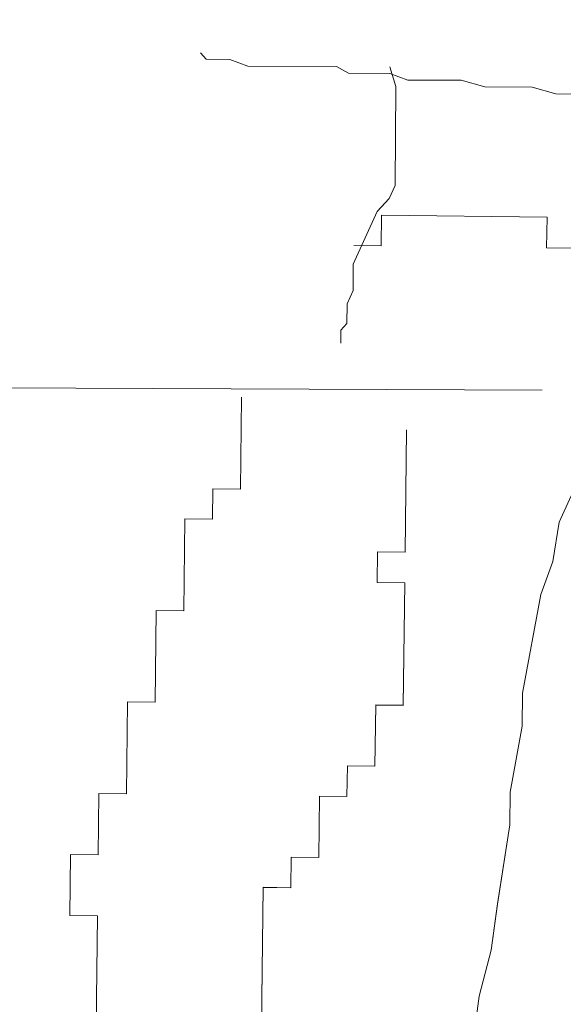
# Model space of a CAD drawing. Units: inches. Extents: x -466983 to 1020, y 324 to 318697.
# Tile 77 of 97: x 650.415 to 652.867, y 944.271 to 948.713. Entities that reach past the tile are written whole.
import ezdxf

# ---------------------------------------------------------------- set-up
doc = ezdxf.new("R2010")
doc.units = ezdxf.units.IN
doc.header["$MEASUREMENT"] = 0
doc.layers.add('A-FLOR-PATT', color=252, linetype='Continuous', lineweight=13)
doc.layers.add('A-FURN', color=8, linetype='Continuous', lineweight=18)

# ---------------------------------------------------------------- blocks, each defined once
blk = doc.blocks.new('L Shaped Sofa')
at = {"ltscale": 2}
for p, q in [((2404.6561, 739.9002), (2404.7023, 743.6789)), ((2402.8786, 740.7957), (2402.9297, 741.175)), ((2406.0202, 740.1355), (2406.0325, 741.1431)), ((2402.7787, 740.4166), (2402.8786, 740.7957)), ((2402.7276, 740.0374), (2402.7787, 740.4166)), ((2406.2471, 740.1327), (2406.0202, 740.1355)), ((2406.2409, 739.6289), (2406.2471, 740.1327)), ((2402.626, 739.3872), (2402.7276, 740.0374)), ((2404.4262, 739.6511), (2404.4293, 739.903)), ((2404.4293, 739.903), (2404.6561, 739.9002)), ((2404.1932, 739.15), (2404.1994, 739.6538)), ((2404.1994, 739.6538), (2404.4262, 739.6511)), ((2406.0079, 739.1279), (2406.0141, 739.6317)), ((2406.0141, 739.6317), (2406.2409, 739.6289)), ((2402.6243, 739.1161), (2402.626, 739.3872)), ((2403.9633, 738.9009), (2403.9664, 739.1528)), ((2403.9664, 739.1528), (2404.1932, 739.15)), ((2405.7718, 738.3749), (2405.7811, 739.1306)), ((2405.7811, 739.1306), (2406.0079, 739.1279)), ((2402.5234, 738.5744), (2402.6243, 739.1161)), ((2403.7303, 738.3998), (2403.7365, 738.9037)), ((2403.7365, 738.9037), (2403.9633, 738.9009)), ((2402.5218, 738.3034), (2402.5234, 738.5744)), ((2403.4912, 737.395), (2403.5035, 738.4026)), ((2403.5035, 738.4026), (2403.7303, 738.3998)), ((2405.5358, 737.6219), (2405.545, 738.3777)), ((2405.545, 738.3777), (2405.7718, 738.3749)), ((2402.3704, 737.4908), (2402.5218, 738.3034)), ((2405.2997, 736.869), (2405.3089, 737.6247)), ((2405.3089, 737.6247), (2405.5358, 737.6219)), ((2402.2712, 737.2202), (2402.3704, 737.4908)), ((2403.718, 737.3922), (2403.4912, 737.395)), ((2403.7149, 737.1403), (2403.718, 737.3922)), ((2402.2204, 736.8951), (2402.2712, 737.2202)), ((2403.4758, 736.1354), (2403.4881, 737.143)), ((2403.4881, 737.143), (2403.7149, 737.1403)), ((2402.1214, 736.6787), (2402.2204, 736.8951)), ((2405.0698, 736.6198), (2405.0729, 736.8717)), ((2405.0729, 736.8717), (2405.2997, 736.869)), ((2404.8337, 735.8669), (2404.843, 736.6226)), ((2404.843, 736.6226), (2405.0698, 736.6198)), ((2402.3601, 735.8101), (2406.8981, 735.7888)), ((2404.0162, 735.3144), (2404.0168, 735.4228)), ((2403.967, 735.2604), (2404.0162, 735.3144)), ((2403.966, 735.0978), (2403.967, 735.2604)), ((2403.9166, 734.9896), (2403.966, 735.0978)), ((2403.9152, 734.7727), (2403.9166, 734.9896)), ((2403.7174, 734.3399), (2403.9152, 734.7727)), ((2402.0963, 734.6406), (2402.3231, 734.6378)), ((2402.3231, 734.6378), (2402.3201, 734.3859)), ((2403.6811, 734.3692), (2403.6842, 734.6212)), ((2403.6842, 734.6212), (2403.911, 734.6184)), ((2402.3201, 734.3859), (2403.6811, 734.3692)), ((2403.6192, 734.2319), (2403.7174, 734.3399)), ((2403.5697, 734.1237), (2403.6192, 734.2319)), ((2403.5647, 733.3105), (2403.5697, 734.1237)), ((2401.7596, 733.3732), (2402.2476, 733.3709)), ((2402.2476, 733.3709), (2402.4424, 733.3157)), ((2402.4424, 733.3157), (2402.8328, 733.3139)), ((2402.8328, 733.3139), (2403.0276, 733.2588)), ((2403.6125, 733.1476), (2403.5647, 733.3105)), ((2403.0276, 733.2588), (2403.4668, 733.2567)), ((2403.4668, 733.2567), (2403.6129, 733.2018)), ((2403.6129, 733.2018), (2403.9544, 733.2002)), ((2403.9544, 733.2002), (2404.0517, 733.1455)), ((2404.0517, 733.1455), (2404.7836, 733.1421)), ((2404.7836, 733.1421), (2404.9297, 733.0872)), ((2404.9297, 733.0872), (2405.1248, 733.0863)), ((2405.1248, 733.0863), (2405.1733, 733.0318))]:
    blk.add_line(p, q, dxfattribs=at)

msp = doc.modelspace()

# ---------------------------------------------------------------- hatches: boundary and pattern name
at = {"layer": 'A-FLOR-PATT', "transparency": 33554572}
h = msp.add_hatch(dxfattribs=at)
h.set_pattern_fill('ANSI37', color=256, scale=30)
h.set_pattern_definition([(45, (-1212.4137, -290.035), (-2.6516504, 2.6516504), []), (135, (-1212.4137, -290.035), (-2.6516504, -2.6516504), [])])
h.paths.add_polyline_path([(901.8057, 1075.9377), (900.6144, 1075.9377), (900.6144, 1065.3856), (899.391, 1065.3856), (898.0911, 1065.3856), (892.8356, 1058.7098, -0.258377), (892.1875, 1058.3509), (879.9848, 1058.3509, -0.20177), (879.4382, 1058.5808), (874.0812, 1065.3856), (872.7813, 1065.3856), (871.5579, 1065.3856), (871.5579, 1075.9377), (813.8057, 1075.9377), (813.8057, 1044.7922), (832.3947, 1044.7922, -0.394795), (848.6602, 1028.5356), (848.6602, 1009.9377), (901.8057, 1009.9377), (901.8057, 1015.9377), (901.3057, 1015.9377), (871.3057, 1015.9377), (871.3057, 1017.2502), (871.3344, 1017.2502, -0.401453), (901.3057, 1045.9377), (901.8057, 1045.9377)])
edge = h.paths.add_edge_path(flags=16)
edge.add_line((847.7731, 1068.9486), (847.7731, 1073.7088))
edge.add_arc((849.2269, 1073.7088), 1.4538, 90, 180, ccw=False)
edge.add_line((849.2269, 1075.1627), (864.4921, 1075.1627))
edge.add_arc((864.4921, 1073.7088), 1.4538, 0, 90, ccw=False)
edge.add_line((865.9459, 1073.7088), (865.9459, 1069.0035))
edge.add_arc((832.6447, 1068.9761), 33.3012, -20.61234, 0.04725, ccw=False)
edge.add_ellipse((856.8595, 1058.48), major_axis=(0, 10.2131), ratio=0.6859192, start_angle=100.00884, end_angle=259.99116, ccw=False)
edge.add_arc((881.0742, 1068.9761), 33.3012, 180.04725, 200.61234, ccw=False)
h.paths.add_polyline_path([(853.1456, 1066.4815), (853.1456, 1066.4534), (853.1463, 1066.4534, 0.433107), (852.9166, 1066.6849), (852.9166, 1066.4534), (853.1456, 1066.4534), (853.1456, 1066.4815), (853.088, 1066.6122, 0.697939), (852.6995, 1066.4534), (852.7003, 1066.4534), (852.7003, 1066.4815), (852.9166, 1067.0012), (852.9166, 1066.6849, -0.396254)], flags=0)
h.paths.add_polyline_path([(861.0187, 1066.4815), (861.0187, 1066.4534), (861.0194, 1066.4534, 0.416404), (860.8024, 1066.6849), (860.8024, 1066.4534), (861.0187, 1066.4534), (861.0187, 1066.4815), (860.9672, 1066.6053, 0.713344), (860.5726, 1066.4534), (860.5734, 1066.4534), (860.5734, 1066.4815), (860.8024, 1067.0012), (860.8024, 1066.6849, -0.379973)], flags=0)
edge = h.paths.add_edge_path(flags=0)
edge.add_spline(control_points=[(861.1298, 1065.7855), (861.4661, 1065.2478), (861.6134, 1065.0161), (861.9833, 1064.3736), (862.1924, 1063.9443), (862.5614, 1063.0391), (862.7212, 1062.5633), (862.9865, 1061.5781), (863.092, 1061.0689), (863.2452, 1060.031), (863.293, 1059.5025), (863.3295, 1058.4409), (863.3181, 1057.9078), (863.2366, 1056.8518), (863.1664, 1056.3289), (862.9695, 1055.308), (862.8427, 1054.8099), (862.5365, 1053.8522), (862.3571, 1053.3927), (861.9514, 1052.5249), (861.7251, 1052.1166), (861.233, 1051.3622), (860.9672, 1051.0162), (860.4048, 1050.3949), (860.1082, 1050.1197), (859.4937, 1049.6461), (859.1758, 1049.4476), (858.5276, 1049.1299), (858.1973, 1049.0107), (857.5315, 1048.8518), (857.1959, 1048.8121), (856.5249, 1048.812), (856.1894, 1048.8515), (855.5236, 1049.0101), (855.1933, 1049.1291), (854.545, 1049.4465), (854.2271, 1049.6449), (853.6124, 1050.1183), (853.3158, 1050.3933), (852.7533, 1051.0143), (852.4874, 1051.3602), (851.9952, 1052.1144), (851.7688, 1052.5225), (851.3629, 1053.3902), (851.1834, 1053.8496), (850.877, 1054.8071), (850.7501, 1055.3051), (850.553, 1056.326), (850.4827, 1056.8488), (850.401, 1057.9048), (850.3895, 1058.4379), (850.4257, 1059.4995), (850.4734, 1060.0281), (850.6265, 1061.066), (850.7318, 1061.5753), (850.9969, 1062.5605), (851.1567, 1063.0365), (851.5254, 1063.9418), (851.7345, 1064.3712), (852.1056, 1065.0164), (852.2544, 1065.2503), (852.6082, 1065.7335)], knot_values=[3.915332, 3.915332, 3.915332, 3.915332, 4.013468, 4.013468, 4.175532, 4.175532, 4.337596, 4.337596, 4.49966, 4.49966, 4.661724, 4.661724, 4.823788, 4.823788, 4.985852, 4.985852, 5.147916, 5.147916, 5.30998, 5.30998, 5.472044, 5.472044, 5.634109, 5.634109, 5.796173, 5.796173, 5.958237, 5.958237, 6.120301, 6.120301, 6.282365, 6.282365, 6.444429, 6.444429, 6.606493, 6.606493, 6.768557, 6.768557, 6.930621, 6.930621, 7.092685, 7.092685, 7.254749, 7.254749, 7.416813, 7.416813, 7.578878, 7.578878, 7.740942, 7.740942, 7.903006, 7.903006, 8.06507, 8.06507, 8.227134, 8.227134, 8.389198, 8.389198, 8.551262, 8.551262, 8.65037, 8.65037, 8.65037, 8.65037], degree=3, periodic=0)
edge.add_line((852.6421, 1065.7855), (861.1298, 1065.7855))
edge = h.paths.add_edge_path(flags=0)
edge.add_ellipse((856.8496, 1057.7432), major_axis=(0, 7.7921), ratio=0.687861, start_angle=0, end_angle=360)
h.paths.add_polyline_path([(848.8634, 1069.3891), (848.8634, 1073.9605, -0.414214), (849.9538, 1075.0508), (863.7652, 1075.0508, -0.414214), (864.8555, 1073.9605), (864.8555, 1069.3891, -0.388936), (864.5237, 1069.027, -0.043561), (849.1953, 1069.027, -0.388936)], flags=0)
h.paths.add_polyline_path([(853.1006, 1068.1122, -1), (852.6775, 1068.1122, -1)], flags=0)
edge = h.paths.add_edge_path(flags=0)
edge.add_ellipse((856.8595, 1057.3378), major_axis=(0, 2.207), ratio=0.657164, start_angle=0, end_angle=360)
h.paths.add_polyline_path([(861.0415, 1068.1122, -1), (860.6184, 1068.1122, -1)], flags=0)
edge = h.paths.add_edge_path()
edge.add_line((573.9537, 1057.3412), (573.9537, 1075.9377))
edge.add_line((573.9537, 1075.9377), (558.7308, 1075.9377))
edge.add_line((558.7308, 1075.9377), (558.7308, 1065.3856))
edge.add_line((558.7308, 1065.3856), (557.5074, 1065.3856))
edge.add_line((557.5074, 1065.3856), (556.2075, 1065.3856))
edge.add_line((556.2075, 1065.3856), (550.952, 1058.7098))
edge.add_arc((550.3039, 1059.1155), 0.7646, 270, 327.9483, ccw=False)
edge.add_line((550.3039, 1058.3509), (538.1012, 1058.3509))
edge.add_arc((538.1012, 1059.1155), 0.7646, 224.3704, 270, ccw=False)
edge.add_line((537.5546, 1058.5808), (532.1976, 1065.3856))
edge.add_line((532.1976, 1065.3856), (530.8977, 1065.3856))
edge.add_line((530.8977, 1065.3856), (529.6743, 1065.3856))
edge.add_line((529.6743, 1065.3856), (529.6743, 1075.9377))
edge.add_line((529.6743, 1075.9377), (520.8057, 1075.9377))
edge.add_line((520.8057, 1075.9377), (520.8057, 1045.9377))
edge.add_line((520.8057, 1045.9377), (521.3057, 1045.9377))
edge.add_arc((521.3057, 1015.9377), 30, 2.50749, 90, ccw=False)
edge.add_line((551.277, 1017.2502), (551.3057, 1017.2502))
edge.add_line((551.3057, 1017.2502), (551.3057, 1015.9377))
edge.add_line((551.3057, 1015.9377), (520.8057, 1015.9377))
edge.add_line((520.8057, 1015.9377), (520.8057, 1009.9377))
edge.add_line((520.8057, 1009.9377), (559.1913, 1010.4022))
edge.add_arc((559.1913, 1011.856), 1.4538, 180, 270, ccw=False)
edge.add_line((557.7375, 1011.856), (557.7375, 1016.5613))
edge.add_arc((591.0386, 1016.5888), 33.3012, 159.38766, 180.04725, ccw=False)
edge.add_ellipse((566.8239, 1027.0848), major_axis=(0, 10.2131), ratio=0.6859192, start_angle=280.00884, end_angle=439.99116, ccw=False)
edge.add_arc((542.6091, 1016.5888), 33.3012, 0.04725, 20.61234, ccw=False)
edge.add_line((575.9103, 1016.6162), (575.9103, 1011.856))
edge.add_arc((574.4565, 1011.856), 1.4538, -90, 0, ccw=False)
edge.add_line((574.4565, 1010.4022), (608.8057, 1009.9377))
edge.add_line((608.8057, 1009.9377), (608.8057, 1041.0857))
edge.add_line((608.8057, 1041.0857), (590.2179, 1041.0857))
edge.add_arc((590.775, 1057.9074), 16.8309, 181.92775, 268.10321, ccw=False)
edge = h.paths.add_edge_path()
edge.add_ellipse((494.2443, 583.6204), major_axis=(0, 10.2131), ratio=0.6859192, start_angle=280.00884, end_angle=439.99116, ccw=False)
edge.add_arc((470.0296, 573.1243), 33.3012, 0.04725, 20.61234, ccw=False)
edge.add_line((503.3307, 573.1518), (503.3307, 568.3916))
edge.add_arc((501.8769, 568.3916), 1.4538, -90, 0, ccw=False)
edge.add_line((501.8769, 566.9377), (539.8057, 566.9377))
edge.add_line((539.8057, 566.9377), (539.8057, 572.9377))
edge.add_line((539.8057, 572.9377), (539.3057, 572.9377))
edge.add_line((539.3057, 572.9377), (509.3057, 572.9377))
edge.add_line((509.3057, 572.9377), (509.3057, 574.2502))
edge.add_line((509.3057, 574.2502), (509.3344, 574.2502))
edge.add_arc((539.3057, 572.9377), 30, 90, 177.49251, ccw=False)
edge.add_line((539.3057, 602.9377), (539.8057, 602.9377))
edge.add_line((539.8057, 602.9377), (539.8057, 626.9377))
edge.add_line((539.8057, 626.9377), (531.7718, 626.9377))
edge.add_line((531.7718, 626.9377), (531.7718, 616.3856))
edge.add_line((531.7718, 616.3856), (530.5484, 616.3856))
edge.add_line((530.5484, 616.3856), (529.2485, 616.3856))
edge.add_line((529.2485, 616.3856), (523.7105, 609.3509))
edge.add_line((523.7105, 609.3509), (510.7766, 609.3509))
edge.add_line((510.7766, 609.3509), (505.2386, 616.3856))
edge.add_line((505.2386, 616.3856), (503.9387, 616.3856))
edge.add_line((503.9387, 616.3856), (502.7153, 616.3856))
edge.add_line((502.7153, 616.3856), (502.7153, 626.9377))
edge.add_line((502.7153, 626.9377), (481.6983, 626.9377))
edge.add_line((481.6983, 626.9377), (481.6983, 610.995))
edge.add_arc((467.2703, 611.4728), 14.4359, 271.92775, 358.10321, ccw=False)
edge.add_line((467.7559, 597.0451), (451.8057, 597.0451))
edge.add_line((451.8057, 597.0451), (451.8057, 584.4035))
edge.add_line((451.8057, 584.4035), (451.8057, 566.9377))
edge.add_line((451.8057, 566.9377), (486.6117, 566.9377))
edge.add_arc((486.6117, 568.3916), 1.4538, 180, 270, ccw=False)
edge.add_line((485.1579, 568.3916), (485.1579, 573.0969))
edge.add_arc((518.4591, 573.1243), 33.3012, 159.38766, 180.04725, ccw=False)
h.paths.add_polyline_path([(836.2609, 1020.7328), (879.8898, 1020.7328), (879.8898, 1039.3902), (836.2609, 1039.3902)], flags=25)
h.paths.add_polyline_path([(549.9851, 1036.7492), (593.614, 1036.7492), (593.614, 1055.4065), (549.9851, 1055.4065)], flags=24)
h.paths.add_polyline_path([(475.123, 595.5959), (518.752, 595.5959), (518.752, 614.2532), (475.123, 614.2532)], flags=24)
h = msp.add_hatch(dxfattribs=at)
h.set_pattern_fill('ANSI37', color=256, scale=20)
h.set_pattern_definition([(45, (-1212.4137, -290.035), (-1.767767, 1.767767), []), (135, (-1212.4137, -290.035), (-1.767767, -1.767767), [])])
h.paths.add_polyline_path([(809.8057, 870.9377), (809.8057, 888.1519), (806.9985, 888.1519), (802.6624, 888.1519), (789.3832, 888.1519), (786.2846, 888.1519, -0.414214), (785.4991, 888.9374), (785.4991, 900.1959), (785.4991, 908.4696, -0.414214), (786.8082, 909.7787, -0.414214), (785.4991, 911.0878), (785.4991, 929.1015, -0.414214), (786.8082, 930.4106, -0.414214), (785.4991, 931.7197), (785.4991, 931.9039, -0.414214), (784.19, 930.5948), (766.7223, 930.5948, -0.412359), (765.4132, 931.8956, -0.413741), (764.1145, 930.5782), (744.5781, 930.422, -0.416556), (743.7864, 931.2075), (743.7864, 933.5153), (742.2154, 933.5153), (742.2154, 952.024, -0.001344), (743.7864, 952.1998), (743.7864, 953.9377), (678.5915, 953.9377), (678.5915, 951.1305), (678.5915, 946.7945), (678.5915, 933.5153), (678.5915, 930.4166, -0.414214), (677.806, 929.6312), (666.5475, 929.6312), (658.2738, 929.6312, -0.414214), (656.9647, 930.9403, -0.414214), (655.6556, 929.6312), (637.6419, 929.6312, -0.414214), (636.3328, 930.9403, -0.414214), (635.0237, 929.6312), (634.8395, 929.6312, -0.414214), (636.1486, 928.322), (636.1486, 910.8544, -0.412359), (634.8478, 909.5452, -0.413741), (636.1653, 908.2466), (636.3214, 888.7102, -0.416556), (635.5359, 887.9184), (633.2281, 887.9184), (633.2281, 886.3475), (614.7194, 886.3475, -0.001344), (614.5436, 887.9184), (612.8057, 887.9184), (612.8057, 834.9377), (612.8057, 752.9377), (612.8057, 748.9377), (612.8057, 697.9377), (654.8057, 697.9377), (654.8057, 701.9377), (715.8057, 701.9377), (715.8057, 737.4353), (774.2918, 737.4353), (774.2918, 795.9377), (809.8057, 795.9377)])
h.paths.add_polyline_path([(679.2761, 849.5757, 0.102523), (682.1475, 849.2608, -0.080461), (694.5428, 849.7725, -0.283899), (694.4822, 849.0082, 0.136605), (694.4068, 848.8103, -0.030441), (694.5428, 846.8929), (694.5428, 842.6198), (694.5428, 838.3466, -0.028219), (694.4246, 836.5684), (694.425, 836.5684, 0.196187), (694.4456, 836.2708, -0.302897), (694.5428, 835.467, -0.080461), (682.1475, 835.9787, 0.102523), (679.2761, 835.6638, -0.58611), (678.6457, 836.0169), (678.6457, 849.2227, -0.58611)], flags=16)
h.paths.add_polyline_path([(679.5173, 848.6515, 0.699597), (679.476, 848.6342, 1.20716), (679.1935, 848.7422, 0.010621)], flags=0)
h.paths.add_polyline_path([(679.4923, 836.5608, -0.013798), (679.9178, 836.6594, -0.071703), (682.8533, 837.1434, -0.165743), (682.1665, 839.1006), (682.1665, 842.6094), (682.1665, 846.0603, -0.240616), (683.4733, 848.6767, -0.068263), (693.9295, 849.0082), (693.7875, 848.7083), (693.7875, 849.0228, 0.067332), (683.4733, 848.6767, 0.240616), (682.1665, 846.0603), (682.1665, 842.6094), (682.1665, 839.1006, 0.23459), (683.461, 836.5513, 0.068093), (693.7875, 836.1955), (693.7875, 836.5104), (693.9296, 836.2102, -0.077215), (682.2421, 836.7815, 0.086627), (679.5283, 836.5701, -0.628402), (679.5029, 836.5735), (679.5029, 836.6071, 0.910458)], flags=0)
h.paths.add_polyline_path([(679.476, 848.6364), (679.2069, 848.647), (679.2069, 836.5718, 0.913566), (679.3645, 836.5861), (679.476, 836.5824)], flags=0)
h.paths.add_polyline_path([(679.2761, 829.8604, 0.102523), (682.1475, 829.5455, -0.080461), (694.5428, 830.0572, -0.283899), (694.4822, 829.2929, 0.136605), (694.4068, 829.095, -0.030441), (694.5428, 827.1776), (694.5428, 822.9045), (694.5428, 818.6314, -0.028219), (694.4246, 816.8531), (694.425, 816.8532, 0.196187), (694.4456, 816.5555, -0.302897), (694.5428, 815.7517, -0.080461), (682.1475, 816.2635, 0.102523), (679.2761, 815.9485, -0.58611), (678.6457, 816.3016), (678.6457, 829.5074, -0.58611)], flags=16)
h.paths.add_polyline_path([(679.5173, 828.9362, 0.699597), (679.476, 828.9189, 1.20716), (679.1935, 829.0269, 0.010621)], flags=0)
h.paths.add_polyline_path([(679.4923, 816.8456, -0.013798), (679.9178, 816.9441, -0.071703), (682.8533, 817.4281, -0.165743), (682.1665, 819.3853), (682.1665, 822.8941), (682.1665, 826.345, -0.240616), (683.4733, 828.9614, -0.068263), (693.9295, 829.2929), (693.7875, 828.9931), (693.7875, 829.3076, 0.067332), (683.4733, 828.9614, 0.240616), (682.1665, 826.345), (682.1665, 822.8941), (682.1665, 819.3853, 0.23459), (683.461, 816.836, 0.068093), (693.7875, 816.4802), (693.7875, 816.7952), (693.9296, 816.4949, -0.077215), (682.2421, 817.0662, 0.086627), (679.5283, 816.8549, -0.628402), (679.5029, 816.8582), (679.5029, 816.8918, 0.910458)], flags=0)
h.paths.add_polyline_path([(679.476, 828.9211), (679.2069, 828.9317), (679.2069, 816.8565, 0.913566), (679.3645, 816.8708), (679.476, 816.8671)], flags=0)
h.paths.add_polyline_path([(679.2761, 810.1451, 0.102523), (682.1475, 809.8302, -0.080461), (694.5428, 810.342, -0.3023), (694.4466, 809.5394, 0.10023), (694.4058, 809.3878, -0.03057), (694.5428, 807.4623), (694.5428, 803.1892), (694.5428, 798.9161, -0.03057), (694.4058, 796.9906, 0.10023), (694.4466, 796.839, -0.3023), (694.5428, 796.0365, -0.080461), (682.1475, 796.5482, 0.102523), (679.2761, 796.2333, -0.58611), (678.6457, 796.5863), (678.6457, 809.7921, -0.58611)], flags=16)
h.paths.add_polyline_path([(679.5173, 809.2417, 0.699597), (679.476, 809.2244, 1.20716), (679.1935, 809.3324, 0.010621)], flags=0)
h.paths.add_polyline_path([(679.4923, 797.151, -0.013798), (679.9178, 797.2496, -0.071703), (682.8533, 797.7336, -0.165743), (682.1665, 799.6908), (682.1665, 803.1996), (682.1665, 806.6505, -0.239349), (683.461, 809.2577, -0.072465), (694.4468, 809.5405, 0.197932), (694.425, 809.2405), (693.7875, 809.2985), (693.7875, 809.6135, 0.068093), (683.461, 809.2577, 0.239349), (682.1665, 806.6505), (682.1665, 803.1996), (682.1665, 799.6908, 0.235854), (683.4733, 797.1323, 0.067332), (693.7875, 796.7861), (693.7875, 797.1006), (694.425, 797.1586, 0.197932), (694.4468, 796.8586, -0.080419), (682.1557, 797.3795, 0.083867), (679.5283, 797.1603, -0.628402), (679.5029, 797.1637), (679.5029, 797.1973, 0.910458)], flags=0)
h.paths.add_polyline_path([(679.2069, 809.2372), (679.2069, 797.162, 0.913566), (679.3645, 797.1763), (679.476, 797.1726), (679.476, 809.2266)], flags=0)
h.paths.add_polyline_path([(695.3643, 853.2989), (728.2231, 853.2989), (728.2231, 771.1519), (695.3643, 771.1519)], flags=16)
h.paths.add_polyline_path([(696.0215, 852.6417), (727.5659, 852.6417), (727.5659, 771.809), (696.0215, 771.809)], flags=0)
h.paths.add_polyline_path([(679.2761, 788.7869, 0.102523), (682.1475, 788.472, -0.080461), (694.5428, 788.9837, -0.3023), (694.4466, 788.1812, 0.10023), (694.4058, 788.0296, -0.03057), (694.5428, 786.1041), (694.5428, 781.831), (694.5428, 777.5578, -0.03057), (694.4058, 775.6323, 0.10023), (694.4466, 775.4808, -0.3023), (694.5428, 774.6782, -0.080461), (682.1475, 775.19, 0.102523), (679.2761, 774.875, -0.58611), (678.6457, 775.2281), (678.6457, 788.4339, -0.58611)], flags=16)
h.paths.add_polyline_path([(679.5173, 787.8834, 0.699597), (679.476, 787.8662, 1.20716), (679.1935, 787.9742, 0.010621)], flags=0)
h.paths.add_polyline_path([(679.4923, 775.7928, -0.013798), (679.9178, 775.8914, -0.071703), (682.8533, 776.3753, -0.165743), (682.1665, 778.3325), (682.1665, 781.8414), (682.1665, 785.2922, -0.239349), (683.461, 787.8995, -0.072465), (694.4468, 788.1823, 0.197932), (694.425, 787.8823), (693.7875, 787.9403), (693.7875, 788.2553, 0.068093), (683.461, 787.8995, 0.239349), (682.1665, 785.2922), (682.1665, 781.8414), (682.1665, 778.3325, 0.235854), (683.4733, 775.7741, 0.067332), (693.7875, 775.4279), (693.7875, 775.7424), (694.425, 775.8004, 0.197932), (694.4468, 775.5004, -0.080419), (682.1557, 776.0212, 0.083867), (679.5283, 775.8021, -0.628402), (679.5029, 775.8054), (679.5029, 775.8391, 0.910458)], flags=0)
h.paths.add_polyline_path([(679.2069, 787.8789), (679.2069, 775.8038, 0.913566), (679.3645, 775.818), (679.476, 775.8144), (679.476, 787.8684)], flags=0)
h.paths.add_polyline_path([(704.641, 854.1204, -0.080461), (705.1527, 866.5157, 0.102523), (704.8378, 869.3871, -0.58611), (705.1908, 870.0174), (718.3966, 870.0174, -0.58611), (718.7496, 869.3871, 0.102523), (718.4347, 866.5157, -0.080461), (718.9465, 854.1204, -0.3023), (718.1439, 854.2166, 0.10023), (717.9924, 854.2574, -0.03057), (716.0668, 854.1204), (711.7937, 854.1204), (707.5206, 854.1204, -0.03057), (705.5951, 854.2574, 0.10023), (705.4435, 854.2166, -0.3023)], flags=16)
h.paths.add_polyline_path([(717.8462, 869.1459, 0.699597), (717.8289, 869.1872, 1.20716), (717.9369, 869.4697, 0.010621)], flags=0)
h.paths.add_polyline_path([(705.4631, 854.2164, -0.080419), (705.984, 866.5074, 0.083867), (705.7648, 869.1349, -0.628402), (705.7682, 869.1603), (705.8018, 869.1603, 0.910458), (705.7555, 869.1709, -0.013798), (705.8541, 868.7454, -0.071703), (706.3381, 865.8099, -0.165743), (708.2953, 866.4967), (711.8041, 866.4967), (715.255, 866.4967, -0.239349), (717.8622, 865.2022, -0.072465), (718.145, 854.2164, 0.197932), (717.845, 854.2382), (717.903, 854.8757), (718.218, 854.8757, 0.068093), (717.8622, 865.2022, 0.239349), (715.255, 866.4967), (711.8041, 866.4967), (708.2953, 866.4967, 0.235854), (705.7368, 865.1898, 0.067332), (705.3906, 854.8757), (705.7051, 854.8757), (705.7631, 854.2382, 0.197932)], flags=16)
h.paths.add_polyline_path([(705.7665, 869.4563, 0.913566), (705.7808, 869.2987), (705.7771, 869.1872), (717.8311, 869.1872), (717.8417, 869.4563)], flags=0)
h.paths.add_polyline_path([(729.0446, 842.6198), (729.0446, 846.8929, -0.03057), (729.1817, 848.8184, 0.10023), (729.1408, 848.9699, -0.3023), (729.0446, 849.7725, -0.080461), (741.4399, 849.2608, 0.102523), (744.3113, 849.5757, -0.58611), (744.9417, 849.2227), (744.9417, 836.0169, -0.58611), (744.3113, 835.6638, 0.102523), (741.4399, 835.9787, -0.080461), (729.0446, 835.467, -0.3023), (729.1408, 836.2696, 0.10023), (729.1817, 836.4211, -0.03057), (729.0446, 838.3466)], flags=16)
h.paths.add_polyline_path([(744.1115, 836.5846, 1.20716), (744.3939, 836.4766, 0.010621), (744.0701, 836.5673, 0.699597)], flags=0)
h.paths.add_polyline_path([(729.1407, 836.2684, 0.197932), (729.1624, 836.5684), (729.7999, 836.5104), (729.7999, 836.1955, 0.068093), (740.1264, 836.5513, 0.239349), (741.4209, 839.1585), (741.4209, 842.6094), (741.4209, 846.1182, 0.235854), (740.1141, 848.6767, 0.067332), (729.7999, 849.0228), (729.7999, 848.7083), (729.1624, 848.6503, 0.197932), (729.1407, 848.9504, -0.080419), (741.4317, 848.4295, 0.083867), (744.0591, 848.6486, -0.628402), (744.0845, 848.6453), (744.0845, 848.6117, 0.910458), (744.0951, 848.6579, -0.013798), (743.6696, 848.5594, -0.071703), (740.7341, 848.0754, -0.165743), (741.4209, 846.1182), (741.4209, 842.6094), (741.4209, 839.1585, -0.239349), (740.1264, 836.5513, -0.072465)], flags=0)
h.paths.add_polyline_path([(729.0446, 830.0572, -0.080461), (741.4399, 829.5455, 0.102523), (744.3113, 829.8604, -0.58611), (744.9417, 829.5074), (744.9417, 816.3016, -0.58611), (744.3113, 815.9485, 0.102523), (741.4399, 816.2635, -0.080461), (729.0446, 815.7517, -0.3023), (729.1408, 816.5543, 0.10023), (729.1817, 816.7058, -0.03057), (729.0446, 818.6314), (729.0446, 822.9045), (729.0446, 827.1776, -0.03057), (729.1817, 829.1031, 0.10023), (729.1408, 829.2547, -0.3023)], flags=16)
h.paths.add_polyline_path([(744.1115, 816.8693, 1.20716), (744.3939, 816.7613, 0.010621), (744.0701, 816.852, 0.699597)], flags=0)
h.paths.add_polyline_path([(729.1407, 829.2351, -0.080419), (741.4317, 828.7142, 0.083867), (744.0591, 828.9334, -0.628402), (744.0845, 828.93), (744.0845, 828.8964, 0.910458), (744.0951, 828.9427, -0.013798), (743.6696, 828.8441, -0.071703), (740.7341, 828.3601, -0.165743), (741.4209, 826.4029), (741.4209, 822.8941), (741.4209, 819.4432, -0.239349), (740.1264, 816.836, -0.072465), (729.1407, 816.5531, 0.197932), (729.1624, 816.8532), (729.7999, 816.7952), (729.7999, 816.4802, 0.068093), (740.1264, 816.836, 0.239349), (741.4209, 819.4432), (741.4209, 822.8941), (741.4209, 826.4029, 0.235854), (740.1141, 828.9614, 0.067332), (729.7999, 829.3076), (729.7999, 828.9931), (729.1624, 828.9351, 0.197932)], flags=16)
h.paths.add_polyline_path([(729.0446, 810.342, -0.080461), (741.4399, 809.8302, 0.102523), (744.3113, 810.1451, -0.58611), (744.9417, 809.7921), (744.9417, 796.5863, -0.58611), (744.3113, 796.2333, 0.102523), (741.4399, 796.5482, -0.080461), (729.0446, 796.0365, -0.283899), (729.1052, 796.8007, 0.136605), (729.1806, 796.9987, -0.030441), (729.0446, 798.9161), (729.0446, 803.1892), (729.0446, 807.4623, -0.028219), (729.1628, 809.2406), (729.1624, 809.2405, 0.196187), (729.1418, 809.5382, -0.302897)], flags=16)
h.paths.add_polyline_path([(744.1115, 797.1748, 1.20716), (744.3939, 797.0668, 0.010621), (744.0701, 797.1575, 0.699597)], flags=0)
h.paths.add_polyline_path([(741.3453, 809.0275, 0.086627), (744.0591, 809.2388, -0.628402), (744.0845, 809.2355), (744.0845, 809.2019, 0.910458), (744.0951, 809.2481, -0.013798), (743.6696, 809.1496, -0.071703), (740.7341, 808.6656, -0.165743), (741.4209, 806.7084), (741.4209, 803.1996), (741.4209, 799.7487, -0.240616), (740.1141, 797.1323, -0.068263), (729.658, 796.8008), (729.7999, 797.1006), (729.7999, 796.7861, 0.067332), (740.1141, 797.1323, 0.240616), (741.4209, 799.7487), (741.4209, 803.1996), (741.4209, 806.7084, 0.23459), (740.1264, 809.2577, 0.068093), (729.7999, 809.6135), (729.7999, 809.2985), (729.6578, 809.5988, -0.077215)], flags=0)
h.paths.add_polyline_path([(704.641, 770.3304, -0.283899), (705.4053, 770.2697, 0.136605), (705.6032, 770.1944, -0.030441), (707.5206, 770.3304), (711.7937, 770.3304), (716.0668, 770.3304, -0.028219), (717.8451, 770.2122), (717.845, 770.2126, 0.196187), (718.1427, 770.2331, -0.302897), (718.9465, 770.3304, -0.080461), (718.4347, 757.9351, 0.102523), (718.7496, 755.0637, -0.58611), (718.3966, 754.4333), (705.1908, 754.4333, -0.58611), (704.8378, 755.0637, 0.102523), (705.1527, 757.9351, -0.080461)], flags=16)
h.paths.add_polyline_path([(705.762, 755.3048, 0.699597), (705.7793, 755.2635, 1.20716), (705.6713, 754.9811, 0.010621)], flags=0)
h.paths.add_polyline_path([(705.4053, 769.717), (705.7051, 769.5751), (705.3906, 769.5751, 0.067332), (705.7368, 759.2609, 0.240616), (708.3532, 757.954), (711.8041, 757.954), (715.3129, 757.954, 0.23459), (717.8622, 759.2485, 0.068093), (718.218, 769.5751), (717.903, 769.5751), (718.2033, 769.7172, -0.077215), (717.632, 758.0297, 0.086627), (717.8433, 755.3159, -0.628402), (717.84, 755.2904), (717.8064, 755.2904, 0.910458), (717.8526, 755.2799, -0.013798), (717.7541, 755.7053, -0.071703), (717.2701, 758.6409, -0.165743), (715.3129, 757.954), (711.8041, 757.954), (708.3532, 757.954, -0.240616), (705.7368, 759.2609, -0.068263)], flags=0)
h.paths.add_polyline_path([(729.0446, 788.9837, -0.080461), (741.4399, 788.472, 0.102523), (744.3113, 788.7869, -0.58611), (744.9417, 788.4339), (744.9417, 775.2281, -0.58611), (744.3113, 774.875, 0.102523), (741.4399, 775.19, -0.080461), (729.0446, 774.6782, -0.283899), (729.1052, 775.4425, 0.136605), (729.1806, 775.6405, -0.030441), (729.0446, 777.5578), (729.0446, 781.831), (729.0446, 786.1041, -0.028219), (729.1628, 787.8823), (729.1624, 787.8823, 0.196187), (729.1418, 788.1799, -0.302897)], flags=16)
h.paths.add_polyline_path([(744.1115, 775.8165, 1.20716), (744.3939, 775.7086, 0.010621), (744.0701, 775.7993, 0.699597)], flags=0)
h.paths.add_polyline_path([(741.3453, 787.6692, 0.086627), (744.0591, 787.8806, -0.628402), (744.0845, 787.8773), (744.0845, 787.8437, 0.910458), (744.0951, 787.8899, -0.013798), (743.6696, 787.7913, -0.071703), (740.7341, 787.3074, -0.165743), (741.4209, 785.3502), (741.4209, 781.8414), (741.4209, 778.3905, -0.240616), (740.1141, 775.7741, -0.068263), (729.658, 775.4425), (729.7999, 775.7424), (729.7999, 775.4279, 0.067332), (740.1141, 775.7741, 0.240616), (741.4209, 778.3905), (741.4209, 781.8414), (741.4209, 785.3502, 0.23459), (740.1264, 787.8995, 0.068093), (729.7999, 788.2553), (729.7999, 787.9403), (729.6578, 788.2405, -0.077215)], flags=0)
h.paths.add_polyline_path([(744.1115, 848.6364), (744.1115, 836.5824), (744.3805, 836.5718), (744.3805, 848.647, 0.913566), (744.2229, 848.6327)], flags=0)
h.paths.add_polyline_path([(744.2229, 828.9174), (744.1115, 828.9211), (744.1115, 816.8671), (744.3805, 816.8565), (744.3805, 828.9317, 0.913566)], flags=0)
h.paths.add_polyline_path([(717.8311, 755.2635), (705.7771, 755.2635), (705.7665, 754.9945), (717.8417, 754.9945, 0.913566), (717.8274, 755.1521)], flags=0)
h.paths.add_polyline_path([(744.2229, 809.2229), (744.1115, 809.2266), (744.1115, 797.1726), (744.3805, 797.162), (744.3805, 809.2372, 0.913566)], flags=0)
h.paths.add_polyline_path([(744.1115, 787.8684), (744.1115, 775.8144), (744.3805, 775.8038), (744.3805, 787.8789, 0.913566), (744.2229, 787.8647)], flags=0)
h.paths.add_polyline_path([(678.8774, 877.1228), (737.6127, 877.1228), (737.6127, 899.5116), (678.8774, 899.5116)], flags=24)

# ---------------------------------------------------------------- linework, layer by layer
at = {"layer": 'A-FURN', "ltscale": 2}
for p, q in [((651.2564, 948.534), (651.2298, 948.5639)), ((651.2564, 948.534), (651.2298, 948.5639)), ((651.2564, 948.534), (651.2298, 948.5639)), ((651.2564, 948.534), (651.2298, 948.5639)), ((651.2564, 948.534), (651.2298, 948.5639)), ((651.2564, 948.534), (651.2298, 948.5639)), ((651.3634, 948.5335), (651.2564, 948.534)), ((651.3634, 948.5335), (651.2564, 948.534)), ((651.3634, 948.5335), (651.2564, 948.534)), ((651.3634, 948.5335), (651.2564, 948.534)), ((651.3634, 948.5335), (651.2564, 948.534)), ((651.3634, 948.5335), (651.2564, 948.534)), ((651.4435, 948.5034), (651.3634, 948.5335)), ((651.4435, 948.5034), (651.3634, 948.5335)), ((651.4435, 948.5034), (651.3634, 948.5335)), ((651.4435, 948.5034), (651.3634, 948.5335)), ((651.4435, 948.5034), (651.3634, 948.5335)), ((651.4435, 948.5034), (651.3634, 948.5335)), ((651.8447, 948.5016), (651.4435, 948.5034)), ((651.8447, 948.5016), (651.4435, 948.5034)), ((651.8447, 948.5016), (651.4435, 948.5034)), ((651.8447, 948.5016), (651.4435, 948.5034)), ((651.8447, 948.5016), (651.4435, 948.5034)), ((651.8447, 948.5016), (651.4435, 948.5034)), ((651.898, 948.4716), (651.8447, 948.5016)), ((651.898, 948.4716), (651.8447, 948.5016)), ((651.898, 948.4716), (651.8447, 948.5016)), ((651.898, 948.4716), (651.8447, 948.5016)), ((651.898, 948.4716), (651.8447, 948.5016)), ((651.898, 948.4716), (651.8447, 948.5016)), ((652.0855, 948.5004), (652.1117, 948.4111)), ((652.0855, 948.5004), (652.1117, 948.4111)), ((652.0855, 948.5004), (652.1117, 948.4111)), ((652.0855, 948.5004), (652.1117, 948.4111)), ((652.0855, 948.5004), (652.1117, 948.4111)), ((652.0855, 948.5004), (652.1117, 948.4111)), ((652.0853, 948.4707), (651.898, 948.4716)), ((652.0853, 948.4707), (651.898, 948.4716)), ((652.0853, 948.4707), (651.898, 948.4716)), ((652.0853, 948.4707), (651.898, 948.4716)), ((652.0853, 948.4707), (651.898, 948.4716)), ((652.0853, 948.4707), (651.898, 948.4716)), ((652.1654, 948.4406), (652.0853, 948.4707)), ((652.1654, 948.4406), (652.0853, 948.4707)), ((652.1654, 948.4406), (652.0853, 948.4707)), ((652.1654, 948.4406), (652.0853, 948.4707)), ((652.1654, 948.4406), (652.0853, 948.4707)), ((652.1654, 948.4406), (652.0853, 948.4707)), ((652.1117, 948.4111), (652.1089, 947.9653)), ((652.1117, 948.4111), (652.1089, 947.9653)), ((652.1117, 948.4111), (652.1089, 947.9653)), ((652.1117, 948.4111), (652.1089, 947.9653)), ((652.1117, 948.4111), (652.1089, 947.9653)), ((652.1117, 948.4111), (652.1089, 947.9653)), ((652.4061, 948.4395), (652.1654, 948.4406)), ((652.4061, 948.4395), (652.1654, 948.4406)), ((652.4061, 948.4395), (652.1654, 948.4406)), ((652.4061, 948.4395), (652.1654, 948.4406)), ((652.4061, 948.4395), (652.1654, 948.4406)), ((652.4061, 948.4395), (652.1654, 948.4406)), ((652.5129, 948.4093), (652.4061, 948.4395)), ((652.5129, 948.4093), (652.4061, 948.4395)), ((652.5129, 948.4093), (652.4061, 948.4395)), ((652.5129, 948.4093), (652.4061, 948.4395)), ((652.5129, 948.4093), (652.4061, 948.4395)), ((652.5129, 948.4093), (652.4061, 948.4395)), ((652.7269, 948.4083), (652.5129, 948.4093)), ((652.7269, 948.4083), (652.5129, 948.4093)), ((652.7269, 948.4083), (652.5129, 948.4093)), ((652.7269, 948.4083), (652.5129, 948.4093)), ((652.7269, 948.4083), (652.5129, 948.4093)), ((652.7269, 948.4083), (652.5129, 948.4093)), ((652.8337, 948.378), (652.7269, 948.4083)), ((652.8337, 948.378), (652.7269, 948.4083)), ((652.8337, 948.378), (652.7269, 948.4083)), ((652.8337, 948.378), (652.7269, 948.4083)), ((652.8337, 948.378), (652.7269, 948.4083)), ((652.8337, 948.378), (652.7269, 948.4083)), ((653.1012, 948.3768), (652.8337, 948.378)), ((653.1012, 948.3768), (652.8337, 948.378)), ((653.1012, 948.3768), (652.8337, 948.378)), ((653.1012, 948.3768), (652.8337, 948.378)), ((653.1012, 948.3768), (652.8337, 948.378)), ((653.1012, 948.3768), (652.8337, 948.378)), ((652.1089, 947.9653), (652.0818, 947.906)), ((652.1089, 947.9653), (652.0818, 947.906)), ((652.1089, 947.9653), (652.0818, 947.906)), ((652.1089, 947.9653), (652.0818, 947.906)), ((652.1089, 947.9653), (652.0818, 947.906)), ((652.1089, 947.9653), (652.0818, 947.906)), ((652.0818, 947.906), (652.028, 947.8468)), ((652.0818, 947.906), (652.028, 947.8468)), ((652.0818, 947.906), (652.028, 947.8468)), ((652.0818, 947.906), (652.028, 947.8468)), ((652.0818, 947.906), (652.028, 947.8468)), ((652.0818, 947.906), (652.028, 947.8468)), ((652.028, 947.8468), (651.9195, 947.6095)), ((652.028, 947.8468), (651.9195, 947.6095)), ((652.028, 947.8468), (651.9195, 947.6095)), ((652.028, 947.8468), (651.9195, 947.6095)), ((652.028, 947.8468), (651.9195, 947.6095)), ((652.028, 947.8468), (651.9195, 947.6095)), ((652.0479, 947.8307), (652.0462, 947.6926)), ((652.0479, 947.8307), (652.0462, 947.6926)), ((652.0479, 947.8307), (652.0462, 947.6926)), ((652.0479, 947.8307), (652.0462, 947.6926)), ((652.0479, 947.8307), (652.0462, 947.6926)), ((652.0479, 947.8307), (652.0462, 947.6926)), ((652.794, 947.8216), (652.0479, 947.8307)), ((652.794, 947.8216), (652.0479, 947.8307)), ((652.794, 947.8216), (652.0479, 947.8307)), ((652.794, 947.8216), (652.0479, 947.8307)), ((652.794, 947.8216), (652.0479, 947.8307)), ((652.794, 947.8216), (652.0479, 947.8307)), ((652.7923, 947.6835), (652.794, 947.8216)), ((652.7923, 947.6835), (652.794, 947.8216)), ((652.7923, 947.6835), (652.794, 947.8216)), ((652.7923, 947.6835), (652.794, 947.8216)), ((652.7923, 947.6835), (652.794, 947.8216)), ((652.7923, 947.6835), (652.794, 947.8216)), ((652.0462, 947.6926), (651.9218, 947.6941)), ((652.0462, 947.6926), (651.9218, 947.6941)), ((652.0462, 947.6926), (651.9218, 947.6941)), ((652.0462, 947.6926), (651.9218, 947.6941)), ((652.0462, 947.6926), (651.9218, 947.6941)), ((652.0462, 947.6926), (651.9218, 947.6941)), ((652.9167, 947.682), (652.7923, 947.6835)), ((652.9167, 947.682), (652.7923, 947.6835)), ((652.9167, 947.682), (652.7923, 947.6835)), ((652.9167, 947.682), (652.7923, 947.6835)), ((652.9167, 947.682), (652.7923, 947.6835)), ((652.9167, 947.682), (652.7923, 947.6835)), ((651.9195, 947.6095), (651.9188, 947.4906)), ((651.9195, 947.6095), (651.9188, 947.4906)), ((651.9195, 947.6095), (651.9188, 947.4906)), ((651.9195, 947.6095), (651.9188, 947.4906)), ((651.9195, 947.6095), (651.9188, 947.4906)), ((651.9195, 947.6095), (651.9188, 947.4906)), ((651.9188, 947.4906), (651.8917, 947.4313)), ((651.9188, 947.4906), (651.8917, 947.4313)), ((651.9188, 947.4906), (651.8917, 947.4313)), ((651.9188, 947.4906), (651.8917, 947.4313)), ((651.9188, 947.4906), (651.8917, 947.4313)), ((651.9188, 947.4906), (651.8917, 947.4313)), ((651.8917, 947.4313), (651.8911, 947.3422)), ((651.8917, 947.4313), (651.8911, 947.3422)), ((651.8917, 947.4313), (651.8911, 947.3422)), ((651.8917, 947.4313), (651.8911, 947.3422)), ((651.8917, 947.4313), (651.8911, 947.3422)), ((651.8917, 947.4313), (651.8911, 947.3422)), ((651.8911, 947.3422), (651.8642, 947.3126)), ((651.8911, 947.3422), (651.8642, 947.3126)), ((651.8911, 947.3422), (651.8642, 947.3126)), ((651.8911, 947.3422), (651.8642, 947.3126)), ((651.8911, 947.3422), (651.8642, 947.3126)), ((651.8911, 947.3422), (651.8642, 947.3126)), ((651.8642, 947.3126), (651.8638, 947.2531)), ((651.8642, 947.3126), (651.8638, 947.2531)), ((651.8642, 947.3126), (651.8638, 947.2531)), ((651.8642, 947.3126), (651.8638, 947.2531)), ((651.8642, 947.3126), (651.8638, 947.2531)), ((651.8642, 947.3126), (651.8638, 947.2531)), ((652.7721, 947.0408), (650.2843, 947.0525)), ((652.7721, 947.0408), (650.2843, 947.0525)), ((652.7721, 947.0408), (650.2843, 947.0525)), ((652.7721, 947.0408), (650.2843, 947.0525)), ((652.7721, 947.0408), (650.2843, 947.0525)), ((652.7721, 947.0408), (650.2843, 947.0525)), ((651.416, 947.0097), (651.4109, 946.5954)), ((651.416, 947.0097), (651.4109, 946.5954)), ((651.416, 947.0097), (651.4109, 946.5954)), ((651.416, 947.0097), (651.4109, 946.5954)), ((651.416, 947.0097), (651.4109, 946.5954)), ((651.416, 947.0097), (651.4109, 946.5954)), ((652.1604, 946.8625), (652.1537, 946.3101)), ((652.1604, 946.8625), (652.1537, 946.3101)), ((652.1604, 946.8625), (652.1537, 946.3101)), ((652.1604, 946.8625), (652.1537, 946.3101)), ((652.1604, 946.8625), (652.1537, 946.3101)), ((652.1604, 946.8625), (652.1537, 946.3101)), ((651.2866, 946.5969), (651.2849, 946.4588)), ((651.2866, 946.5969), (651.2849, 946.4588)), ((651.2866, 946.5969), (651.2849, 946.4588)), ((651.2866, 946.5969), (651.2849, 946.4588)), ((651.2866, 946.5969), (651.2849, 946.4588)), ((651.2866, 946.5969), (651.2849, 946.4588)), ((651.4109, 946.5954), (651.2866, 946.5969)), ((651.4109, 946.5954), (651.2866, 946.5969)), ((651.4109, 946.5954), (651.2866, 946.5969)), ((651.4109, 946.5954), (651.2866, 946.5969)), ((651.4109, 946.5954), (651.2866, 946.5969)), ((651.4109, 946.5954), (651.2866, 946.5969)), ((652.9029, 946.5646), (652.8487, 946.446)), ((652.9029, 946.5646), (652.8487, 946.446)), ((652.9029, 946.5646), (652.8487, 946.446)), ((652.9029, 946.5646), (652.8487, 946.446)), ((652.9029, 946.5646), (652.8487, 946.446)), ((652.9029, 946.5646), (652.8487, 946.446)), ((651.1605, 946.4603), (651.1555, 946.046)), ((651.1605, 946.4603), (651.1555, 946.046)), ((651.1605, 946.4603), (651.1555, 946.046)), ((651.1605, 946.4603), (651.1555, 946.046)), ((651.1605, 946.4603), (651.1555, 946.046)), ((651.1605, 946.4603), (651.1555, 946.046)), ((651.2849, 946.4588), (651.1605, 946.4603)), ((651.2849, 946.4588), (651.1605, 946.4603)), ((651.2849, 946.4588), (651.1605, 946.4603)), ((651.2849, 946.4588), (651.1605, 946.4603)), ((651.2849, 946.4588), (651.1605, 946.4603)), ((651.2849, 946.4588), (651.1605, 946.4603)), ((652.8487, 946.446), (652.8208, 946.2678)), ((652.8487, 946.446), (652.8208, 946.2678)), ((652.8487, 946.446), (652.8208, 946.2678)), ((652.8487, 946.446), (652.8208, 946.2678)), ((652.8487, 946.446), (652.8208, 946.2678)), ((652.8487, 946.446), (652.8208, 946.2678)), ((652.0293, 946.3116), (652.0276, 946.1735)), ((652.0293, 946.3116), (652.0276, 946.1735)), ((652.0293, 946.3116), (652.0276, 946.1735)), ((652.0293, 946.3116), (652.0276, 946.1735)), ((652.0293, 946.3116), (652.0276, 946.1735)), ((652.0293, 946.3116), (652.0276, 946.1735)), ((652.1537, 946.3101), (652.0293, 946.3116)), ((652.1537, 946.3101), (652.0293, 946.3116)), ((652.1537, 946.3101), (652.0293, 946.3116)), ((652.1537, 946.3101), (652.0293, 946.3116)), ((652.1537, 946.3101), (652.0293, 946.3116)), ((652.1537, 946.3101), (652.0293, 946.3116)), ((652.8208, 946.2678), (652.7664, 946.1194)), ((652.8208, 946.2678), (652.7664, 946.1194)), ((652.8208, 946.2678), (652.7664, 946.1194)), ((652.8208, 946.2678), (652.7664, 946.1194)), ((652.8208, 946.2678), (652.7664, 946.1194)), ((652.8208, 946.2678), (652.7664, 946.1194)), ((652.0276, 946.1735), (652.152, 946.172)), ((652.0276, 946.1735), (652.152, 946.172)), ((652.0276, 946.1735), (652.152, 946.172)), ((652.0276, 946.1735), (652.152, 946.172)), ((652.0276, 946.1735), (652.152, 946.172)), ((652.0276, 946.1735), (652.152, 946.172)), ((652.152, 946.172), (652.1452, 945.6196)), ((652.152, 946.172), (652.1452, 945.6196)), ((652.152, 946.172), (652.1452, 945.6196)), ((652.152, 946.172), (652.1452, 945.6196)), ((652.152, 946.172), (652.1452, 945.6196)), ((652.152, 946.172), (652.1452, 945.6196)), ((652.7664, 946.1194), (652.6834, 945.674)), ((652.7664, 946.1194), (652.6834, 945.674)), ((652.7664, 946.1194), (652.6834, 945.674)), ((652.7664, 946.1194), (652.6834, 945.674)), ((652.7664, 946.1194), (652.6834, 945.674)), ((652.7664, 946.1194), (652.6834, 945.674)), ((651.0311, 946.0475), (651.026, 945.6332)), ((651.0311, 946.0475), (651.026, 945.6332)), ((651.0311, 946.0475), (651.026, 945.6332)), ((651.0311, 946.0475), (651.026, 945.6332)), ((651.0311, 946.0475), (651.026, 945.6332)), ((651.0311, 946.0475), (651.026, 945.6332)), ((651.1555, 946.046), (651.0311, 946.0475)), ((651.1555, 946.046), (651.0311, 946.0475)), ((651.1555, 946.046), (651.0311, 946.0475)), ((651.1555, 946.046), (651.0311, 946.0475)), ((651.1555, 946.046), (651.0311, 946.0475)), ((651.1555, 946.046), (651.0311, 946.0475)), ((652.6834, 945.674), (652.6825, 945.5253)), ((652.6834, 945.674), (652.6825, 945.5253)), ((652.6834, 945.674), (652.6825, 945.5253)), ((652.6834, 945.674), (652.6825, 945.5253)), ((652.6834, 945.674), (652.6825, 945.5253)), ((652.6834, 945.674), (652.6825, 945.5253)), ((650.9017, 945.6347), (650.8966, 945.2204)), ((650.9017, 945.6347), (650.8966, 945.2204)), ((650.9017, 945.6347), (650.8966, 945.2204)), ((650.9017, 945.6347), (650.8966, 945.2204)), ((650.9017, 945.6347), (650.8966, 945.2204)), ((650.9017, 945.6347), (650.8966, 945.2204)), ((651.026, 945.6332), (650.9017, 945.6347)), ((651.026, 945.6332), (650.9017, 945.6347)), ((651.026, 945.6332), (650.9017, 945.6347)), ((651.026, 945.6332), (650.9017, 945.6347)), ((651.026, 945.6332), (650.9017, 945.6347)), ((651.026, 945.6332), (650.9017, 945.6347)), ((652.0209, 945.6211), (652.0175, 945.3449)), ((652.0209, 945.6211), (652.0175, 945.3449)), ((652.0209, 945.6211), (652.0175, 945.3449)), ((652.0209, 945.6211), (652.0175, 945.3449)), ((652.0209, 945.6211), (652.0175, 945.3449)), ((652.0209, 945.6211), (652.0175, 945.3449)), ((652.1452, 945.6196), (652.0209, 945.6211)), ((652.1452, 945.6196), (652.0209, 945.6211)), ((652.1452, 945.6196), (652.0209, 945.6211)), ((652.1452, 945.6196), (652.0209, 945.6211)), ((652.1452, 945.6196), (652.0209, 945.6211)), ((652.1452, 945.6196), (652.0209, 945.6211)), ((652.6825, 945.5253), (652.6272, 945.2284)), ((652.6825, 945.5253), (652.6272, 945.2284)), ((652.6825, 945.5253), (652.6272, 945.2284)), ((652.6825, 945.5253), (652.6272, 945.2284)), ((652.6825, 945.5253), (652.6272, 945.2284)), ((652.6825, 945.5253), (652.6272, 945.2284)), ((651.8932, 945.3464), (651.8915, 945.2083)), ((651.8932, 945.3464), (651.8915, 945.2083)), ((651.8932, 945.3464), (651.8915, 945.2083)), ((651.8932, 945.3464), (651.8915, 945.2083)), ((651.8932, 945.3464), (651.8915, 945.2083)), ((651.8932, 945.3464), (651.8915, 945.2083)), ((652.0175, 945.3449), (651.8932, 945.3464)), ((652.0175, 945.3449), (651.8932, 945.3464)), ((652.0175, 945.3449), (651.8932, 945.3464)), ((652.0175, 945.3449), (651.8932, 945.3464)), ((652.0175, 945.3449), (651.8932, 945.3464)), ((652.0175, 945.3449), (651.8932, 945.3464)), ((650.7723, 945.222), (650.7689, 944.9458)), ((650.7723, 945.222), (650.7689, 944.9458)), ((650.7723, 945.222), (650.7689, 944.9458)), ((650.7723, 945.222), (650.7689, 944.9458)), ((650.7723, 945.222), (650.7689, 944.9458)), ((650.7723, 945.222), (650.7689, 944.9458)), ((650.8966, 945.2204), (650.7723, 945.222)), ((650.8966, 945.2204), (650.7723, 945.222)), ((650.8966, 945.2204), (650.7723, 945.222)), ((650.8966, 945.2204), (650.7723, 945.222)), ((650.8966, 945.2204), (650.7723, 945.222)), ((650.8966, 945.2204), (650.7723, 945.222)), ((651.7671, 945.2098), (651.7637, 944.9336)), ((651.7671, 945.2098), (651.7637, 944.9336)), ((651.7671, 945.2098), (651.7637, 944.9336)), ((651.7671, 945.2098), (651.7637, 944.9336)), ((651.7671, 945.2098), (651.7637, 944.9336)), ((651.7671, 945.2098), (651.7637, 944.9336)), ((651.8915, 945.2083), (651.7671, 945.2098)), ((651.8915, 945.2083), (651.7671, 945.2098)), ((651.8915, 945.2083), (651.7671, 945.2098)), ((651.8915, 945.2083), (651.7671, 945.2098)), ((651.8915, 945.2083), (651.7671, 945.2098)), ((651.8915, 945.2083), (651.7671, 945.2098)), ((652.6272, 945.2284), (652.6263, 945.0798)), ((652.6272, 945.2284), (652.6263, 945.0798)), ((652.6272, 945.2284), (652.6263, 945.0798)), ((652.6272, 945.2284), (652.6263, 945.0798)), ((652.6272, 945.2284), (652.6263, 945.0798)), ((652.6272, 945.2284), (652.6263, 945.0798)), ((652.6263, 945.0798), (652.5706, 944.7234)), ((652.6263, 945.0798), (652.5706, 944.7234)), ((652.6263, 945.0798), (652.5706, 944.7234)), ((652.6263, 945.0798), (652.5706, 944.7234)), ((652.6263, 945.0798), (652.5706, 944.7234)), ((652.6263, 945.0798), (652.5706, 944.7234)), ((650.6445, 944.9473), (650.6412, 944.6711)), ((650.6445, 944.9473), (650.6412, 944.6711)), ((650.6445, 944.9473), (650.6412, 944.6711)), ((650.6445, 944.9473), (650.6412, 944.6711)), ((650.6445, 944.9473), (650.6412, 944.6711)), ((650.6445, 944.9473), (650.6412, 944.6711)), ((650.7689, 944.9458), (650.6445, 944.9473)), ((650.7689, 944.9458), (650.6445, 944.9473)), ((650.7689, 944.9458), (650.6445, 944.9473)), ((650.7689, 944.9458), (650.6445, 944.9473)), ((650.7689, 944.9458), (650.6445, 944.9473)), ((650.7689, 944.9458), (650.6445, 944.9473)), ((651.6394, 944.9351), (651.6377, 944.797)), ((651.6394, 944.9351), (651.6377, 944.797)), ((651.6394, 944.9351), (651.6377, 944.797)), ((651.6394, 944.9351), (651.6377, 944.797)), ((651.6394, 944.9351), (651.6377, 944.797)), ((651.6394, 944.9351), (651.6377, 944.797)), ((651.7637, 944.9336), (651.6394, 944.9351)), ((651.7637, 944.9336), (651.6394, 944.9351)), ((651.7637, 944.9336), (651.6394, 944.9351)), ((651.7637, 944.9336), (651.6394, 944.9351)), ((651.7637, 944.9336), (651.6394, 944.9351)), ((651.7637, 944.9336), (651.6394, 944.9351)), ((651.5133, 944.7985), (651.488, 942.727)), ((651.5133, 944.7985), (651.488, 942.727)), ((651.5133, 944.7985), (651.488, 942.727)), ((651.5133, 944.7985), (651.488, 942.727)), ((651.5133, 944.7985), (651.488, 942.727)), ((651.5133, 944.7985), (651.488, 942.727)), ((651.6377, 944.797), (651.5133, 944.7985)), ((651.6377, 944.797), (651.5133, 944.7985)), ((651.6377, 944.797), (651.5133, 944.7985)), ((651.6377, 944.797), (651.5133, 944.7985)), ((651.6377, 944.797), (651.5133, 944.7985)), ((651.6377, 944.797), (651.5133, 944.7985)), ((652.5706, 944.7234), (652.5426, 944.5154)), ((652.5706, 944.7234), (652.5426, 944.5154)), ((652.5706, 944.7234), (652.5426, 944.5154)), ((652.5706, 944.7234), (652.5426, 944.5154)), ((652.5706, 944.7234), (652.5426, 944.5154)), ((652.5706, 944.7234), (652.5426, 944.5154)), ((650.6412, 944.6711), (650.7655, 944.6696)), ((650.6412, 944.6711), (650.7655, 944.6696)), ((650.6412, 944.6711), (650.7655, 944.6696)), ((650.6412, 944.6711), (650.7655, 944.6696)), ((650.6412, 944.6711), (650.7655, 944.6696)), ((650.6412, 944.6711), (650.7655, 944.6696)), ((650.7655, 944.6696), (650.7588, 944.1171)), ((650.7655, 944.6696), (650.7588, 944.1171)), ((650.7655, 944.6696), (650.7588, 944.1171)), ((650.7655, 944.6696), (650.7588, 944.1171)), ((650.7655, 944.6696), (650.7588, 944.1171)), ((650.7655, 944.6696), (650.7588, 944.1171)), ((652.5426, 944.5154), (652.4878, 944.3076)), ((652.5426, 944.5154), (652.4878, 944.3076)), ((652.5426, 944.5154), (652.4878, 944.3076)), ((652.5426, 944.5154), (652.4878, 944.3076)), ((652.5426, 944.5154), (652.4878, 944.3076)), ((652.5426, 944.5154), (652.4878, 944.3076)), ((652.4878, 944.3076), (652.4598, 944.0997)), ((652.4878, 944.3076), (652.4598, 944.0997)), ((652.4878, 944.3076), (652.4598, 944.0997)), ((652.4878, 944.3076), (652.4598, 944.0997)), ((652.4878, 944.3076), (652.4598, 944.0997)), ((652.4878, 944.3076), (652.4598, 944.0997))]:
    msp.add_line(p, q, dxfattribs=at)

# ---------------------------------------------------------------- block references
at = {"layer": 'A-FURN', "xscale": 0.5482153745360612, "yscale": 0.5482153745360612, "zscale": 0.5482153745360612, "rotation": 180}
msp.add_blockref('L Shaped Sofa', (1969.7828, 1350.4232), dxfattribs=at)

doc.saveas('drawing.dxf')
